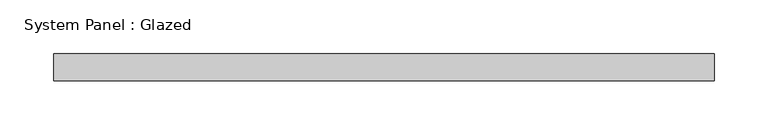
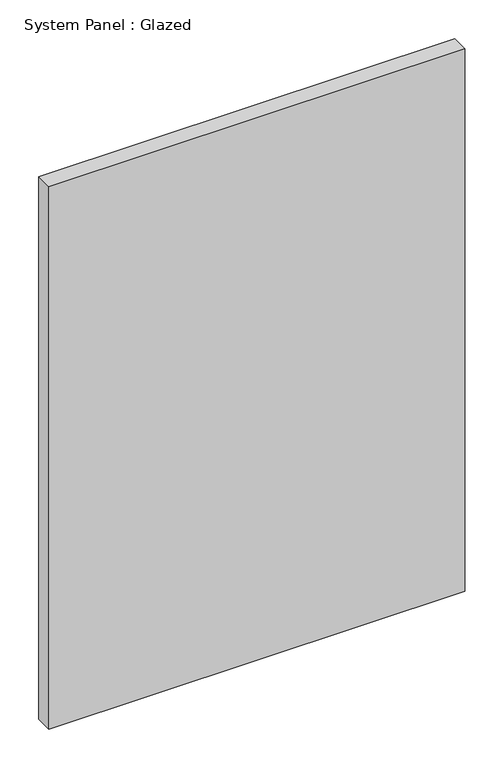
"""IFC4 building model written with IfcOpenShell, lengths in millimetres: plate geometry, System Panel : Glazed."""

from ifc_helpers import new_model, si_unit, origin, origin_with_axes, place, context, project, spatial, polyline, outline, extrude, source, transform, mapped, element, save


def system_panel_glazed_f63241ef(model_context):
    return source(origin(), model_context, "Body", "SweptSolid", [
        extrude(outline(polyline([(307.975, 19.05), (-307.975, 19.05), (-307.975, 44.45), (307.975, 44.45), (307.975, 19.05)])), origin_with_axes(), (0.0, 0.0, 1.0), 849.2180153),
    ])


if __name__ == "__main__":
    model = new_model("IFC4")
    model_context = context("Model", 3, world=origin())
    ifc_project = project(units=[si_unit("LENGTHUNIT", "METRE", prefix="MILLI")], contexts=[model_context])
    site = spatial("IfcSite", under=ifc_project)
    building = spatial("IfcBuilding", under=site)
    placement = place(None, origin())
    system_panel_glazed_shape = system_panel_glazed_f63241ef(model_context)
    element("IfcPlate", 1, ObjectType="System Panel : Glazed", at=placement, inside=building, context=model_context, shape_type="MappedRepresentation", body=[
        mapped(system_panel_glazed_shape, transform((0.0, 0.0, 0.0), x_axis=(1.0, 0.0, 0.0), y_axis=(0.0, 1.0, 0.0), z_axis=(0.0, 0.0, 1.0))),
    ])
    save(model, "model.ifc")

# Revit data of these elements
# Type "System Panel : Glazed"
#   Construction Type Id = "GSP4R"
#   Analytic Construction = "1/8 in Pilkington single glazing"
#   Visual Light Transmittance = 0.9
#   Solar Heat Gain Coefficient = 0.86
#   Heat Transfer Coefficient (U) = 1.18115 BTU/(h·ft²·°F)
#   Define Thermal Properties by = 1
# Element 1 (IfcPlate, "System Panel : Glazed")
#   Materials on its faces: "Glass"
# Materials
#   "Glass": class "Glass", colour RGB 0 128 192, transparency 0.75, Description = "Soda Lime Glass", Cost = 0
